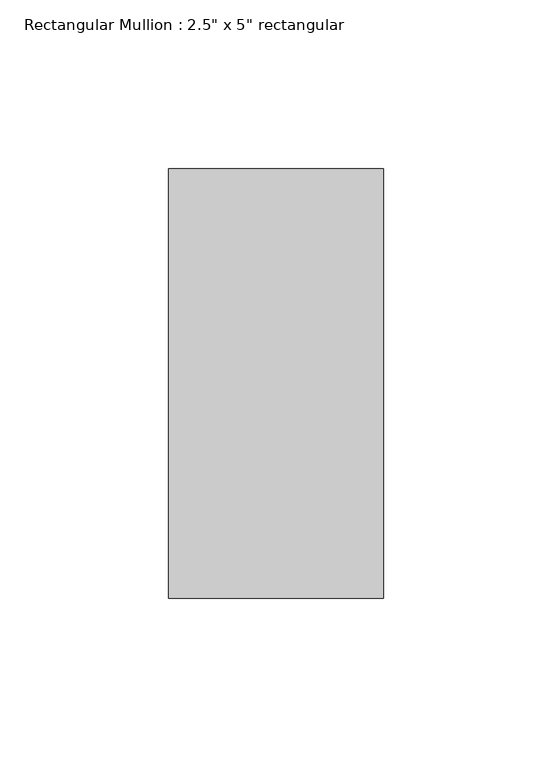
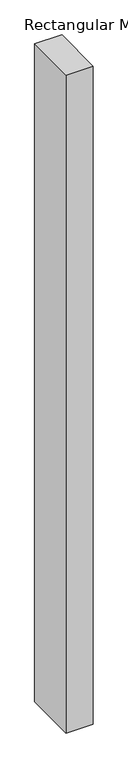
"""IFC4 building model written with IfcOpenShell, lengths in millimetres: member geometry."""

from ifc_helpers import new_model, si_unit, frame, origin, place, context, project, spatial, polyline, outline, extrude, source, transform, mapped, element, save


def member_3d641c1c(model_context):
    return source(origin(), model_context, "Body", "SweptSolid", [
        extrude(outline(polyline([(0.0, 63.5), (0.0, -63.5), (-63.5, -63.5), (-63.5, 63.5), (0.0, 63.5)])), frame((0.0, 0.0, -1629.0255085), z_axis=(0.0, 0.0, 1.0), x_axis=(1.0, 0.0, 0.0)), (0.0, 0.0, 1.0), 1629.0255085),
    ])


if __name__ == "__main__":
    model = new_model("IFC4")
    model_context = context("Model", 3, world=origin())
    ifc_project = project(units=[si_unit("LENGTHUNIT", "METRE", prefix="MILLI")], contexts=[model_context])
    site = spatial("IfcSite", under=ifc_project)
    building = spatial("IfcBuilding", under=site)
    placement = place(None, origin())
    member_shape = member_3d641c1c(model_context)
    element("IfcMember", 1, ObjectType="Rectangular Mullion : 2.5\" x 5\" rectangular", at=placement, inside=building, context=model_context, shape_type="MappedRepresentation", body=[
        mapped(member_shape, transform((0.0, 0.0, 0.0), x_axis=(1.0, 0.0, 0.0), y_axis=(0.0, 1.0, 0.0), z_axis=(0.0, 0.0, 1.0))),
    ])
    save(model, "model.ifc")

# Revit data of these elements
# Type "Rectangular Mullion : 2.5\" x 5\" rectangular"
#   built-in parameter 1007304 = 0.416667 (stored number, unit not read)
#   built-in parameter 1007301 = 0.104167 (stored number, unit not read)
#   built-in parameter 1007300 = 0.104167 (stored number, unit not read)
# Element 1 (IfcMember, "Rectangular Mullion : 2.5\" x 5\" rectangular")
#   Materials on its faces: "Aluminum"
# Materials
#   "Aluminum": class "Metal", colour RGB 247 247 247, transparency 0, Description = "Aluminum 6061", Cost = 0
